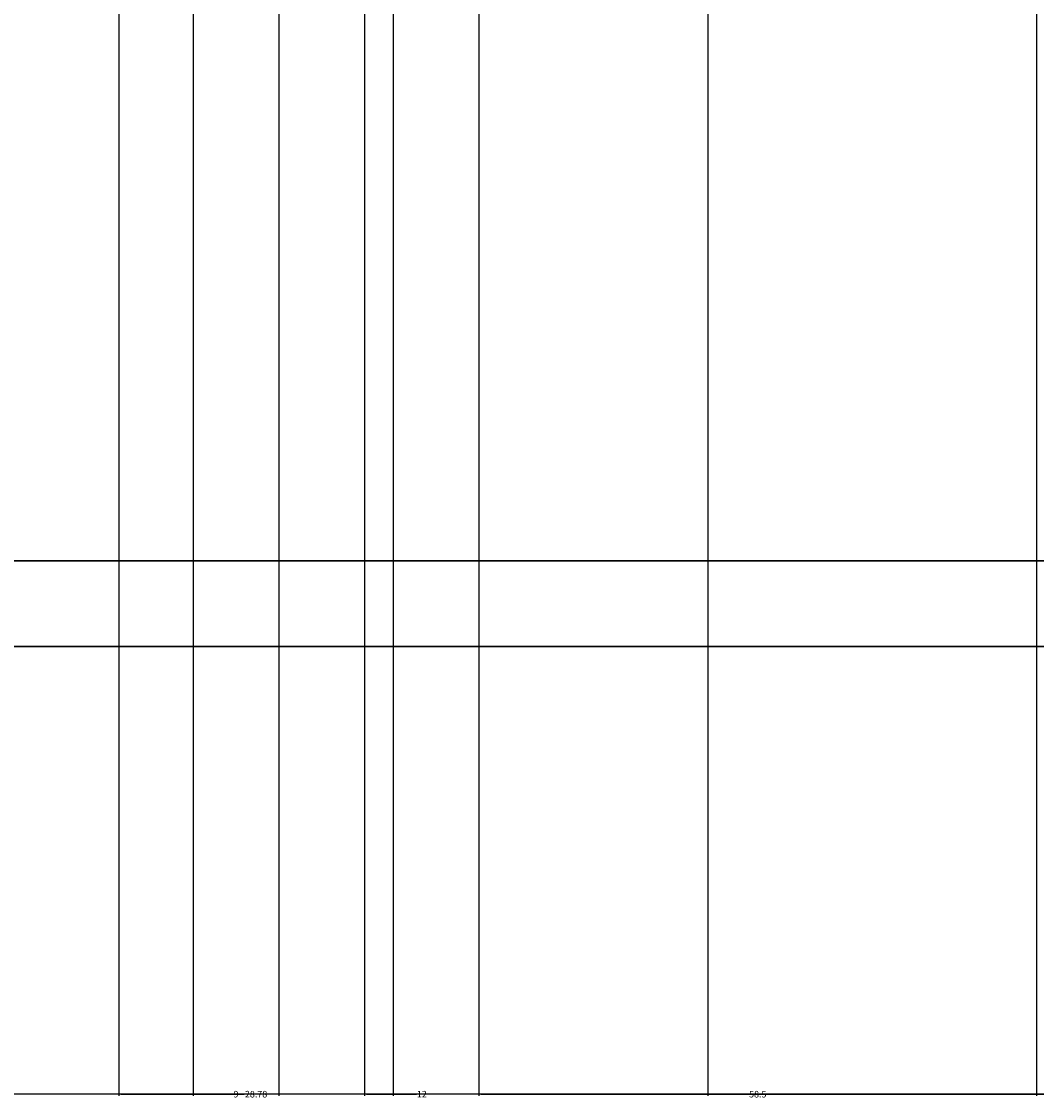
# Model space of a CAD drawing. Units: inches. Extents: x 867 to 1667, y -234 to 788.
# Tile 17 of 42: x 1356 to 1462, y -234 to -121. Entities that reach past the tile are written whole.
import ezdxf

# ---------------------------------------------------------------- set-up
doc = ezdxf.new("R2010")
doc.units = ezdxf.units.IN
doc.header["$MEASUREMENT"] = 0
doc.layers.add('A-ANNO-DIMS', color=2, linetype='Continuous', lineweight=18)
doc.layers.add('A-WALL-SITE', color=8, linetype='Continuous', lineweight=30)
doc.styles.get("Standard").update_dxf_attribs({"font": 'arial.ttf'})
doc.dimstyles.get("Standard").update_dxf_attribs({"dimtxt": 0.6875, "dimasz": 0.18, "dimexe": 0.18, "dimexo": 0.0625, "dimgap": 0.09, "dimtad": 0, "dimdec": 4, "dimzin": 0, "dimdsep": 46, "dimlunit": 4, "dimtxsty": 'Standard', "dimcen": 0.09, "dimadec": 0, "dimazin": 0, "dimtfac": 1, "dimtdec": 4, "dimtofl": 0, "dimtmove": 0, "dimatfit": 3, "dimfxl": 1, "dimtolj": 1, "dimtzin": 0, "dimarcsym": 0})

# ---------------------------------------------------------------- blocks, each defined once
blk = doc.blocks.new('*D23')
at = {"layer": 'A-ANNO-DIMS', "color": 0, "lineweight": -2, "transparency": 16777216}
for p, q in [((1373.89, 623.55), (1373.89, -233.54)), ((1382.89, 623.55), (1382.89, -233.54)), ((1374.07, -233.36), (1378.07, -233.36)), ((1382.71, -233.36), (1378.7, -233.36))]:
    blk.add_line(p, q, dxfattribs=at)
at = {"layer": 'A-ANNO-DIMS', "color": 0, "transparency": 16777216}
for points in [[(1374.07, -233.33), (1374.07, -233.39), (1373.89, -233.36)], [(1382.71, -233.33), (1382.71, -233.39), (1382.89, -233.36)]]:
    blk.add_solid(points, dxfattribs=at)
at = {"layer": 'Defpoints', "color": 0, "transparency": 16777216}
for p in [(1373.89, 623.62), (1382.89, 623.62), (1382.89, -233.36)]:
    blk.add_point(p, dxfattribs=at)
at = {"layer": 'A-ANNO-DIMS', "color": 0, "transparency": 16777216, "insert": (1378.39, -233.36), "char_height": 0.688, "attachment_point": 5}
blk.add_mtext('\\A1;9', dxfattribs=at)
blk = doc.blocks.new('*D27')
at = {"layer": 'A-ANNO-DIMS', "color": 0, "lineweight": -2, "transparency": 16777216}
for p, q in [((1070.89, -55.97), (1070.89, -233.54)), ((1525.26, -186.47), (1525.26, -233.54)), ((1071.07, -233.36), (1296.81, -233.36)), ((1525.08, -233.36), (1299.34, -233.36))]:
    blk.add_line(p, q, dxfattribs=at)
at = {"layer": 'A-ANNO-DIMS', "color": 0, "transparency": 16777216}
for points in [[(1071.07, -233.33), (1071.07, -233.39), (1070.89, -233.36)], [(1525.08, -233.33), (1525.08, -233.39), (1525.26, -233.36)]]:
    blk.add_solid(points, dxfattribs=at)
at = {"layer": 'Defpoints', "color": 0, "transparency": 16777216}
for p in [(1070.89, -55.91), (1525.26, -186.41), (1525.26, -233.36)]:
    blk.add_point(p, dxfattribs=at)
at = {"layer": 'A-ANNO-DIMS', "color": 0, "transparency": 16777216, "insert": (1298.08, -233.36), "char_height": 0.688, "attachment_point": 5}
blk.add_mtext('\\A1;454.4', dxfattribs=at)
blk = doc.blocks.new('*D38')
at = {"layer": 'A-ANNO-DIMS', "color": 0, "lineweight": -2, "transparency": 16777216}
for p, q in [((1403.89, -7.95), (1403.89, -233.54)), ((1559.89, -7.95), (1559.89, -233.54)), ((1404.07, -233.36), (1481.07, -233.36)), ((1559.71, -233.36), (1482.7, -233.36))]:
    blk.add_line(p, q, dxfattribs=at)
at = {"layer": 'A-ANNO-DIMS', "color": 0, "transparency": 16777216}
for points in [[(1404.07, -233.33), (1404.07, -233.39), (1403.89, -233.36)], [(1559.71, -233.33), (1559.71, -233.39), (1559.89, -233.36)]]:
    blk.add_solid(points, dxfattribs=at)
at = {"layer": 'Defpoints', "color": 0, "transparency": 16777216}
for p in [(1403.89, -7.88), (1559.89, -7.88), (1559.89, -233.36)]:
    blk.add_point(p, dxfattribs=at)
at = {"layer": 'A-ANNO-DIMS', "color": 0, "transparency": 16777216, "insert": (1481.89, -233.36), "char_height": 0.688, "attachment_point": 5}
blk.add_mtext('\\A1;156', dxfattribs=at)
blk = doc.blocks.new('*D46')
at = {"layer": 'A-ANNO-DIMS', "color": 0, "lineweight": -2, "transparency": 16777216}
for p, q in [((1256.89, -16.95), (1256.89, -233.54)), ((1394.89, -16.95), (1394.89, -233.54)), ((1257.07, -233.36), (1325.07, -233.36)), ((1394.71, -233.36), (1326.7, -233.36))]:
    blk.add_line(p, q, dxfattribs=at)
at = {"layer": 'A-ANNO-DIMS', "color": 0, "transparency": 16777216}
for points in [[(1257.07, -233.33), (1257.07, -233.39), (1256.89, -233.36)], [(1394.71, -233.33), (1394.71, -233.39), (1394.89, -233.36)]]:
    blk.add_solid(points, dxfattribs=at)
at = {"layer": 'Defpoints', "color": 0, "transparency": 16777216}
for p in [(1256.89, -16.88), (1394.89, -16.88), (1394.89, -233.36)]:
    blk.add_point(p, dxfattribs=at)
at = {"layer": 'A-ANNO-DIMS', "color": 0, "transparency": 16777216, "insert": (1325.89, -233.36), "char_height": 0.688, "attachment_point": 5}
blk.add_mtext('\\A1;138', dxfattribs=at)
blk = doc.blocks.new('*D50')
at = {"layer": 'A-ANNO-DIMS', "color": 0, "lineweight": -2, "transparency": 16777216}
for p, q in [((1211.89, -103.97), (1211.89, -233.54)), ((1427.89, -103.97), (1427.89, -233.54)), ((1212.07, -233.36), (1319.03, -233.36)), ((1427.71, -233.36), (1320.74, -233.36))]:
    blk.add_line(p, q, dxfattribs=at)
at = {"layer": 'A-ANNO-DIMS', "color": 0, "transparency": 16777216}
for points in [[(1212.07, -233.33), (1212.07, -233.39), (1211.89, -233.36)], [(1427.71, -233.33), (1427.71, -233.39), (1427.89, -233.36)]]:
    blk.add_solid(points, dxfattribs=at)
at = {"layer": 'Defpoints', "color": 0, "transparency": 16777216}
for p in [(1211.89, -103.91), (1427.89, -103.91), (1427.89, -233.36)]:
    blk.add_point(p, dxfattribs=at)
at = {"layer": 'A-ANNO-DIMS', "color": 0, "transparency": 16777216, "insert": (1319.89, -233.36), "char_height": 0.688, "attachment_point": 5}
blk.add_mtext('\\A1;216', dxfattribs=at)
blk = doc.blocks.new('*D52')
at = {"layer": 'A-ANNO-DIMS', "color": 0, "lineweight": -2, "transparency": 16777216}
for p, q in [((1391.89, -55.97), (1391.89, -233.54)), ((1403.89, -55.97), (1403.89, -233.54)), ((1392.07, -233.36), (1397.34, -233.36)), ((1403.71, -233.36), (1398.43, -233.36))]:
    blk.add_line(p, q, dxfattribs=at)
at = {"layer": 'A-ANNO-DIMS', "color": 0, "transparency": 16777216}
for points in [[(1392.07, -233.33), (1392.07, -233.39), (1391.89, -233.36)], [(1403.71, -233.33), (1403.71, -233.39), (1403.89, -233.36)]]:
    blk.add_solid(points, dxfattribs=at)
at = {"layer": 'Defpoints', "color": 0, "transparency": 16777216}
for p in [(1391.89, -55.91), (1403.89, -55.91), (1403.89, -233.36)]:
    blk.add_point(p, dxfattribs=at)
at = {"layer": 'A-ANNO-DIMS', "color": 0, "transparency": 16777216, "insert": (1397.89, -233.36), "char_height": 0.688, "attachment_point": 5}
blk.add_mtext('\\A1;12', dxfattribs=at)
blk = doc.blocks.new('*D58')
at = {"layer": 'A-ANNO-DIMS', "color": 0, "lineweight": -2, "transparency": 16777216}
for p, q in [((1403.89, -7.95), (1403.89, -233.54)), ((1462.39, -7.95), (1462.39, -233.54)), ((1404.07, -233.36), (1432.15, -233.36)), ((1462.21, -233.36), (1434.12, -233.36))]:
    blk.add_line(p, q, dxfattribs=at)
at = {"layer": 'A-ANNO-DIMS', "color": 0, "transparency": 16777216}
for points in [[(1404.07, -233.33), (1404.07, -233.39), (1403.89, -233.36)], [(1462.21, -233.33), (1462.21, -233.39), (1462.39, -233.36)]]:
    blk.add_solid(points, dxfattribs=at)
at = {"layer": 'Defpoints', "color": 0, "transparency": 16777216}
for p in [(1403.89, -7.88), (1462.39, -7.88), (1462.39, -233.36)]:
    blk.add_point(p, dxfattribs=at)
at = {"layer": 'A-ANNO-DIMS', "color": 0, "transparency": 16777216, "insert": (1433.14, -233.36), "char_height": 0.688, "attachment_point": 5}
blk.add_mtext('\\A1;58.5', dxfattribs=at)
blk = doc.blocks.new('*D60')
at = {"layer": 'A-ANNO-DIMS', "color": 0, "lineweight": -2, "transparency": 16777216}
for p, q in [((1366.11, 136.05), (1366.11, -233.54)), ((1394.89, 136.05), (1394.89, -233.54)), ((1366.29, -233.36), (1379.24, -233.36)), ((1394.71, -233.36), (1381.75, -233.36))]:
    blk.add_line(p, q, dxfattribs=at)
at = {"layer": 'A-ANNO-DIMS', "color": 0, "transparency": 16777216}
for points in [[(1366.29, -233.33), (1366.29, -233.39), (1366.11, -233.36)], [(1394.71, -233.33), (1394.71, -233.39), (1394.89, -233.36)]]:
    blk.add_solid(points, dxfattribs=at)
at = {"layer": 'Defpoints', "color": 0, "transparency": 16777216}
for p in [(1366.11, 136.12), (1394.89, 136.12), (1394.89, -233.36)]:
    blk.add_point(p, dxfattribs=at)
at = {"layer": 'A-ANNO-DIMS', "color": 0, "transparency": 16777216, "insert": (1380.5, -233.36), "char_height": 0.688, "attachment_point": 5}
blk.add_mtext('\\A1;28.78', dxfattribs=at)

msp = doc.modelspace()

# ---------------------------------------------------------------- linework, layer by layer
at = {"layer": 'A-WALL-SITE'}
for p, q in [((1526.8389, -177.4081), (1006.3882, -177.4081)), ((1211.8866, -177.4081), (1427.8866, -177.4081)), ((1619.8866, -186.4081), (914.8866, -186.4081)), ((1211.8866, -186.4081), (1427.8866, -186.4081))]:
    msp.add_line(p, q, dxfattribs=at)

# ---------------------------------------------------------------- dimensions: what is measured, and where the dimension line sits
at = {"layer": 'A-ANNO-DIMS'}
for base, p1, p2, override, picture, middle in [((1382.8866, -233.3581), (1373.8866, 623.617), (1382.8866, 623.617), {"dimdec": 0, "dimlfac": 1, "dimrnd": 0, "dimzin": 0, "dimdsep": 46, "dimlunit": 2}, '*D23', (1378.3866, -233.3581)), ((1394.8866, -233.3581), (1366.1051, 136.117), (1394.8866, 136.117), {"dimdec": 2, "dimlfac": 1, "dimrnd": 0, "dimzin": 0, "dimdsep": 46, "dimlunit": 2}, '*D60', (1380.4959, -233.3581)), ((1559.8866, -233.3581), (1403.8866, -7.883), (1559.8866, -7.883), {"dimdec": 0, "dimlfac": 1, "dimrnd": 0, "dimzin": 0, "dimdsep": 46, "dimlunit": 2}, '*D38', (1481.8866, -233.3581)), ((1462.3866, -233.3581), (1403.8866, -7.883), (1462.3866, -7.883), {"dimdec": 1, "dimlfac": 1, "dimrnd": 0, "dimzin": 0, "dimdsep": 46, "dimlunit": 2}, '*D58', (1433.1366, -233.3581)), ((1394.8866, -233.3581), (1256.8866, -16.883), (1394.8866, -16.883), {"dimdec": 0, "dimlfac": 1, "dimrnd": 0, "dimzin": 0, "dimdsep": 46, "dimlunit": 2}, '*D46', (1325.8866, -233.3581)), ((1525.2648, -233.3581), (1070.8866, -55.9081), (1525.2648, -186.4081), {"dimdec": 1, "dimlfac": 1, "dimrnd": 0, "dimzin": 0, "dimdsep": 46, "dimlunit": 2}, '*D27', (1298.0757, -233.3581)), ((1403.8866, -233.3581), (1391.8866, -55.9081), (1403.8866, -55.9081), {"dimdec": 0, "dimlfac": 1, "dimrnd": 0, "dimzin": 0, "dimdsep": 46, "dimlunit": 2}, '*D52', (1397.8866, -233.3581)), ((1427.8866, -233.3581), (1211.8866, -103.9081), (1427.8866, -103.9081), {"dimdec": 0, "dimlfac": 1, "dimrnd": 0, "dimzin": 0, "dimdsep": 46, "dimlunit": 2}, '*D50', (1319.8866, -233.3581))]:
    dim = msp.add_linear_dim(base=base, p1=p1, p2=p2, dimstyle='Standard', override=override, dxfattribs=at)
    dim.commit()
    dim.dimension.update_dxf_attribs({"geometry": picture, "text_midpoint": middle})

doc.saveas('drawing.dxf')
